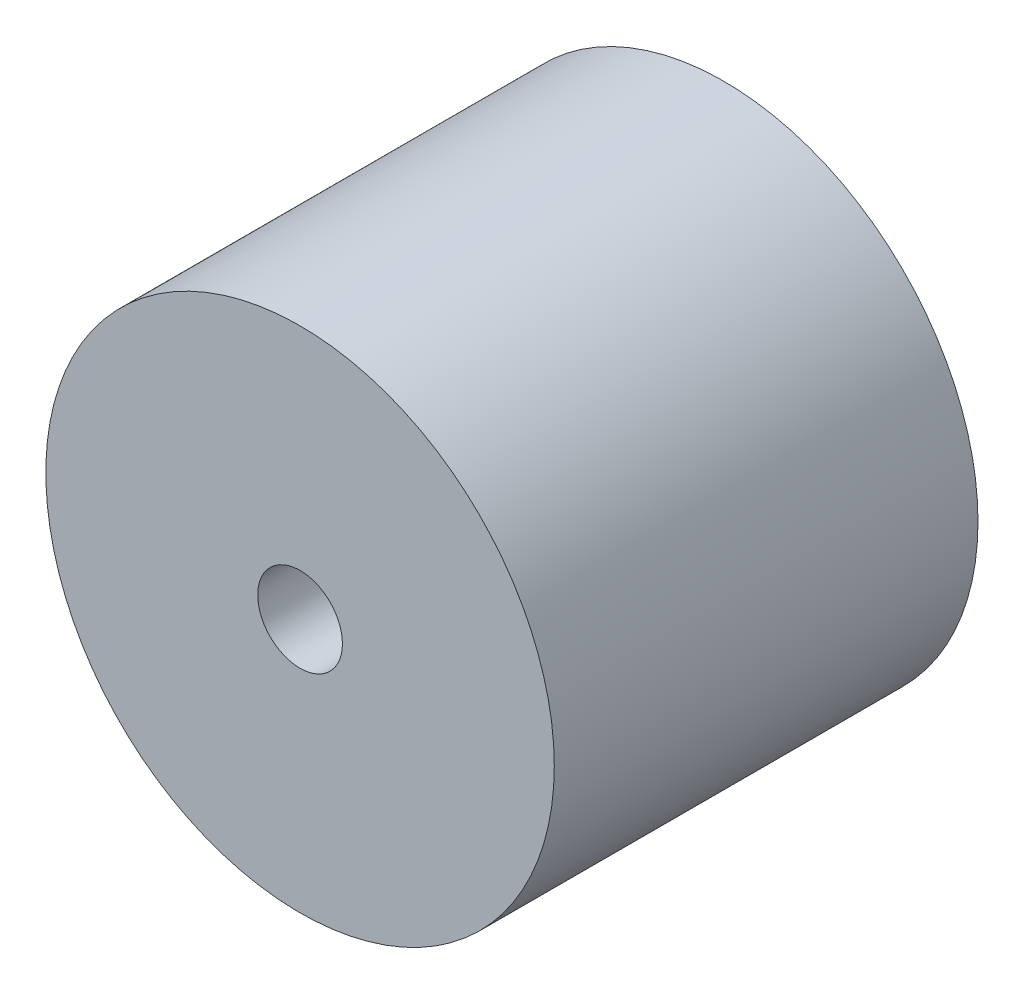
ISO-10303-21;
HEADER;
FILE_DESCRIPTION(('STEP AP214'),'2;1');
FILE_NAME('part.step','',(''),(''),'','','');
FILE_SCHEMA(('AUTOMOTIVE_DESIGN { 1 0 10303 214 1 1 1 1 }'));
ENDSEC;
DATA;
#1=APPLICATION_CONTEXT('core data for automotive mechanical design processes');
#2=APPLICATION_PROTOCOL_DEFINITION('international standard','automotive_design',2000,#1);
#3=PRODUCT_CONTEXT('',#1,'mechanical');
#4=PRODUCT('Part','Part','',(#3));
#5=PRODUCT_RELATED_PRODUCT_CATEGORY('part','',(#4));
#6=PRODUCT_DEFINITION_FORMATION('','',#4);
#7=PRODUCT_DEFINITION_CONTEXT('part definition',#1,'design');
#8=PRODUCT_DEFINITION('design','',#6,#7);
#9=PRODUCT_DEFINITION_SHAPE('','',#8);
#10=(LENGTH_UNIT() NAMED_UNIT(*) SI_UNIT(.MILLI.,.METRE.));
#11=(NAMED_UNIT(*) PLANE_ANGLE_UNIT() SI_UNIT($,.RADIAN.));
#12=(NAMED_UNIT(*) SI_UNIT($,.STERADIAN.) SOLID_ANGLE_UNIT());
#13=UNCERTAINTY_MEASURE_WITH_UNIT(LENGTH_MEASURE(1.E-05),#10,'distance_accuracy_value','');
#14=(GEOMETRIC_REPRESENTATION_CONTEXT(3) GLOBAL_UNCERTAINTY_ASSIGNED_CONTEXT((#13)) GLOBAL_UNIT_ASSIGNED_CONTEXT((#10,
#11,#12)) REPRESENTATION_CONTEXT('',''));
#15=CARTESIAN_POINT('',(0.,0.,0.));
#16=DIRECTION('',(0.,0.,1.));
#17=DIRECTION('',(1.,0.,0.));
#18=AXIS2_PLACEMENT_3D('',#15,#16,#17);
#19=CARTESIAN_POINT('',(0.,0.,15.));
#20=DIRECTION('',(0.,0.,1.));
#21=DIRECTION('',(1.,0.,0.));
#22=AXIS2_PLACEMENT_3D('',#19,#20,#21);
#23=PLANE('',#22);
#24=CARTESIAN_POINT('',(0.,0.,15.));
#25=DIRECTION('',(0.,0.,1.));
#26=DIRECTION('',(1.,0.,0.));
#27=AXIS2_PLACEMENT_3D('',#24,#25,#26);
#28=CIRCLE('',#27,18.);
#29=CARTESIAN_POINT('',(18.,0.,15.));
#30=VERTEX_POINT('',#29);
#31=EDGE_CURVE('E10',#30,#30,#28,.T.);
#32=ORIENTED_EDGE('',*,*,#31,.T.);
#33=EDGE_LOOP('',(#32));
#34=FACE_BOUND('',#33,.T.);
#35=CARTESIAN_POINT('',(0.,0.,15.));
#36=DIRECTION('',(0.,0.,1.));
#37=DIRECTION('',(1.,0.,0.));
#38=AXIS2_PLACEMENT_3D('',#35,#36,#37);
#39=CIRCLE('',#38,3.);
#40=CARTESIAN_POINT('',(3.,0.,15.));
#41=VERTEX_POINT('',#40);
#42=EDGE_CURVE('E53',#41,#41,#39,.T.);
#43=ORIENTED_EDGE('',*,*,#42,.F.);
#44=EDGE_LOOP('',(#43));
#45=FACE_BOUND('',#44,.T.);
#46=ADVANCED_FACE('F43',(#34,#45),#23,.T.);
#47=CARTESIAN_POINT('',(0.,0.,-15.));
#48=DIRECTION('',(0.,0.,1.));
#49=DIRECTION('',(1.,0.,0.));
#50=AXIS2_PLACEMENT_3D('',#47,#48,#49);
#51=PLANE('',#50);
#52=CARTESIAN_POINT('',(0.,0.,-15.));
#53=DIRECTION('',(0.,0.,1.));
#54=DIRECTION('',(1.,0.,0.));
#55=AXIS2_PLACEMENT_3D('',#52,#53,#54);
#56=CIRCLE('',#55,18.);
#57=CARTESIAN_POINT('',(18.,0.,-15.));
#58=VERTEX_POINT('',#57);
#59=EDGE_CURVE('E50',#58,#58,#56,.T.);
#60=ORIENTED_EDGE('',*,*,#59,.F.);
#61=EDGE_LOOP('',(#60));
#62=FACE_BOUND('',#61,.T.);
#63=CARTESIAN_POINT('',(0.,0.,-15.));
#64=DIRECTION('',(0.,0.,1.));
#65=DIRECTION('',(1.,0.,0.));
#66=AXIS2_PLACEMENT_3D('',#63,#64,#65);
#67=CIRCLE('',#66,3.);
#68=CARTESIAN_POINT('',(3.,0.,-15.));
#69=VERTEX_POINT('',#68);
#70=EDGE_CURVE('E57',#69,#69,#67,.T.);
#71=ORIENTED_EDGE('',*,*,#70,.T.);
#72=EDGE_LOOP('',(#71));
#73=FACE_BOUND('',#72,.T.);
#74=ADVANCED_FACE('F67',(#62,#73),#51,.F.);
#75=CARTESIAN_POINT('',(0.,0.,15.));
#76=DIRECTION('',(0.,0.,-1.));
#77=DIRECTION('',(-1.,0.,0.));
#78=AXIS2_PLACEMENT_3D('',#75,#76,#77);
#79=CYLINDRICAL_SURFACE('',#78,18.);
#80=ORIENTED_EDGE('',*,*,#31,.F.);
#81=EDGE_LOOP('',(#80));
#82=FACE_BOUND('',#81,.T.);
#83=ORIENTED_EDGE('',*,*,#59,.T.);
#84=EDGE_LOOP('',(#83));
#85=FACE_BOUND('',#84,.T.);
#86=ADVANCED_FACE('F44',(#82,#85),#79,.T.);
#87=CARTESIAN_POINT('',(0.,0.,15.));
#88=DIRECTION('',(0.,0.,-1.));
#89=DIRECTION('',(-1.,0.,0.));
#90=AXIS2_PLACEMENT_3D('',#87,#88,#89);
#91=CYLINDRICAL_SURFACE('',#90,3.);
#92=ORIENTED_EDGE('',*,*,#42,.T.);
#93=EDGE_LOOP('',(#92));
#94=FACE_BOUND('',#93,.T.);
#95=ORIENTED_EDGE('',*,*,#70,.F.);
#96=EDGE_LOOP('',(#95));
#97=FACE_BOUND('',#96,.T.);
#98=ADVANCED_FACE('F65',(#94,#97),#91,.F.);
#99=CLOSED_SHELL('',(#46,#74,#86,#98));
#100=MANIFOLD_SOLID_BREP('B2',#99);
#101=ADVANCED_BREP_SHAPE_REPRESENTATION('',(#18,#100),#14);
#102=SHAPE_DEFINITION_REPRESENTATION(#9,#101);
ENDSEC;
END-ISO-10303-21;
